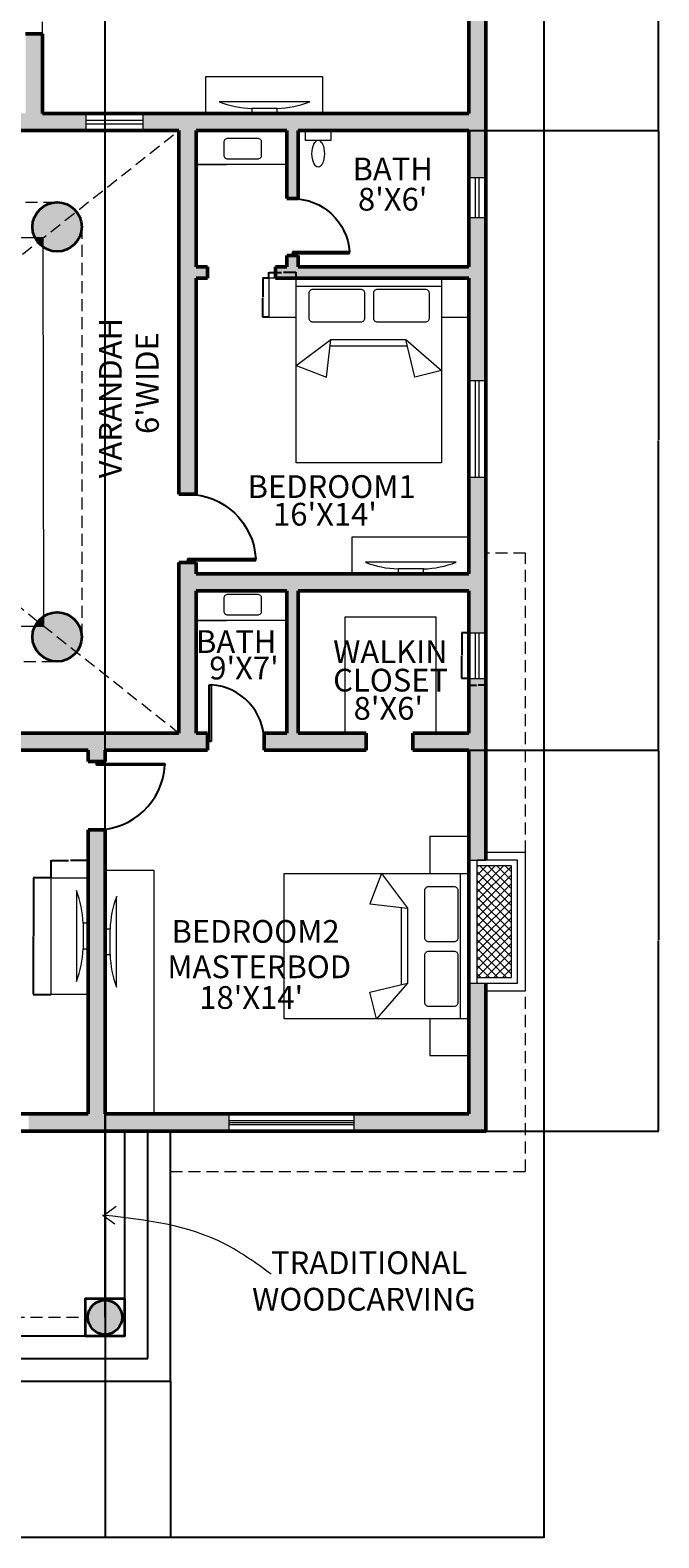
# Model space of a CAD drawing. Units: inches. Extents: x 2743 to 3669, y 1014 to 2282.
# Tile 3 of 5: x 3337 to 3669, y 1014 to 1810. Entities that reach past the tile are written whole.
import ezdxf

# ---------------------------------------------------------------- set-up
doc = ezdxf.new("R2010")
doc.units = ezdxf.units.IN
doc.linetypes.add('DASHED2', pattern=[9.525, 6.35, -3.175])
for name, color, linetype, lineweight in [('A-ANNO-DIMS', 2, 'Continuous', 18), ('A-ANNO-SYMB', 7, 'Continuous', 18), ('A-ANNO-TEXT', 4, 'Continuous', 18), ('A-AREA-IDEN', 4, 'Continuous', 18), ('A-COLS', 7, 'Continuous', 35), ('A-DOOR', 211, 'Continuous', 25), ('A-EQPM', 51, 'Continuous', 18), ('A-FLOR-CASE', 51, 'Continuous', 18), ('A-FLOR-STRS', 7, 'Continuous', 25), ('A-FURN', 111, 'Continuous', 18), ('A-GLAZ', 40, 'Continuous', 20), ('A-GLAZ-PATT', 8, 'Continuous', 13), ('A-ROOF', 7, 'Continuous', 20), ('A-ROOF-OVHD', 8, 'DASHED2', 18), ('A-WALL', 7, 'Continuous', 50), ('A-WALL-OVHD', 8, 'DASHED2', 18)]:
    doc.layers.add(name, color=color, linetype=linetype, lineweight=lineweight)
for name, color, linetype, lineweight, true_color in [('A-COLS-PATT', 47, 'Continuous', 13, 0x726c55), ('A-FLOR-FIXT', 11, 'Continuous', 18, 0xee778f), ('A-WALL-PATT', 47, 'Continuous', 13, 0x726c55)]:
    doc.layers.add(name, color=color, linetype=linetype, lineweight=lineweight, true_color=true_color)
doc.styles.get("Standard").update_dxf_attribs({"font": 'arial.ttf'})
doc.dimstyles.get("Standard").update_dxf_attribs({"dimtxt": 0.18, "dimasz": 0.18, "dimexe": 0.18, "dimexo": 0.0625, "dimgap": 0.09, "dimtad": 0, "dimtih": 1, "dimtoh": 1, "dimdec": 4, "dimzin": 0, "dimdsep": 46, "dimtxsty": 'Standard', "dimcen": 0.09, "dimadec": 0, "dimazin": 0, "dimtfac": 1, "dimtdec": 4, "dimtofl": 0, "dimtmove": 0, "dimatfit": 3, "dimfxl": 1, "dimtolj": 1, "dimtzin": 0, "dimarcsym": 0})

# ---------------------------------------------------------------- blocks, each defined once
blk = doc.blocks.new('DOOR-SINGLE-30IN')
for p, q in [((1, 0), (1, 30)), ((1, 30), (2, 30)), ((2, 30), (2, 0)), ((0, 0), (1, 0)), ((2, 0), (1, 0))]:
    blk.add_line(p, q)
blk.add_arc((0, 0.07), 30, 359.87254, 86.17759)
blk = doc.blocks.new('DOOR-SINGLE-36IN')
for p, q in [((1, 0), (1, 36)), ((1, 36), (2, 36)), ((2, 36), (2, 0)), ((0, 0), (1, 0)), ((2, 0), (1, 0))]:
    blk.add_line(p, q)
blk.add_arc((0, 0.06), 36, 359.91152, 86.81533)
blk = doc.blocks.new('WINDOW-24IN')
for p, q in [((0, 9), (0, 0)), ((24, 9), (24, 0)), ((0, 5.5), (24, 5.5)), ((0, 3.5), (24, 3.5))]:
    blk.add_line(p, q)
blk = doc.blocks.new('BED-DOUBLE')
for p, q in [((4.31, 76.75), (4.31, 0)), ((32.31, 57.96), (48.69, 76.75)), ((48.69, 76.75), (52.23, 62.72)), ((52.23, 62.72), (32.31, 57.96)), ((32.31, 18.34), (32.31, 57.96)), ((35.7, 17.95), (35.72, 58.78)), ((46.06, 0), (32.31, 18.34)), ((52.23, 16.05), (32.31, 18.34)), ((46.06, 0), (52.23, 16.05))]:
    blk.add_line(p, q)
blk.add_lwpolyline([(0, 76.75), (97.38, 76.75), (97.38, 0), (0, 0)], close=True)
for points in [[(7.76, 70.21), (21.16, 70.21, -0.414214), (23.16, 68.21), (23.16, 43, -0.414214), (21.16, 41), (7.76, 41, -0.414214), (5.76, 43), (5.76, 68.21, -0.414214)], [(7.76, 36.18), (21.16, 36.18, -0.414214), (23.16, 34.18), (23.16, 8.97, -0.414214), (21.16, 6.97), (7.76, 6.97, -0.414214), (5.76, 8.97), (5.76, 34.18, -0.414214)]]:
    blk.add_lwpolyline(points, format="xyb", close=True)
blk = doc.blocks.new('NIGHTSTAND')
blk.add_lwpolyline([(0, 0), (20.5, 0), (20.5, 19.45), (0, 19.45)], close=True)
blk = doc.blocks.new('NIGHTSTAND-NARROW')
for p, q in [((14.45, 20.49), (0, 20.49)), ((0, 20.49), (0, 0)), ((14.45, 0), (14.45, 20.49)), ((0, 0), (14.45, 0))]:
    blk.add_line(p, q)
blk = doc.blocks.new('WC')
blk.add_lwpolyline([(0, 13.38), (5.3, 13.38), (5.3, 0), (0, 0)], close=True)
blk.add_ellipse((12.29, 6.69), major_axis=(7.08, 0), ratio=0.464281)
blk = doc.blocks.new('BASIN')
for p, q in [((13.95, 48), (13.95, 0)), ((13.95, 0), (13.95, 16.09))]:
    blk.add_line(p, q)
blk.add_lwpolyline([(2, 34.47), (9.09, 34.47, -0.414214), (11.09, 32.47), (11.09, 16.89, -0.414214), (9.09, 14.89), (2, 14.89, -0.414214), (0, 16.89), (0, 32.47, -0.414214)], format="xyb", close=True)
blk = doc.blocks.new('TV-CONSOLE')
for p, q in [((0, 0), (0, 61.6)), ((0, 61.6), (19.53, 61.6)), ((19.53, 61.6), (19.53, 0)), ((13.42, 54.89), (13.42, 7)), ((19.53, 37.64), (16.89, 37.64)), ((16.89, 37.64), (16.89, 24.26)), ((16.89, 24.26), (19.53, 24.26)), ((19.53, 0), (0, 0))]:
    blk.add_line(p, q)
for centre, radius, start, end in [((-35.21, 36.13), 52.13, 1.66464, 21.09645), ((-35.14, 25.75), 52.05, 338.88993, 358.35791)]:
    blk.add_arc(centre, radius, start, end)
blk = doc.blocks.new('TV-SCREEN')
for p, q in [((6.11, 0), (6.11, 47.89)), ((2.64, 30.63), (0, 30.63)), ((2.64, 17.25), (2.64, 30.63)), ((0, 17.25), (2.64, 17.25))]:
    blk.add_line(p, q)
for centre, radius, start, end in [((54.67, 29.14), 52.05, 158.88993, 178.35791), ((54.74, 18.76), 52.13, 181.66464, 201.09645)]:
    blk.add_arc(centre, radius, start, end)
blk = doc.blocks.new('POST-COURTYARD')
blk.add_circle((13, 13), 13)
blk = doc.blocks.new('POST-SITOUT-OUTER')
blk.add_lwpolyline([(0, 0), (21.09, 0), (21.09, 19.48), (0, 19.48)], close=True)
blk.add_circle((10.55, 9.74), 9.06)
blk = doc.blocks.new('*D34')
at = {"layer": 'A-ANNO-DIMS', "color": 0, "lineweight": -2, "transparency": 16777216}
for p, q in [((3568.73, 1491.96), (3565.02, 1491.96)), ((3565.2, 1491.78), (3565.2, 1480.15)), ((3565.2, 1468.14), (3565.2, 1479.78)), ((3568.73, 1467.96), (3565.02, 1467.96))]:
    blk.add_line(p, q, dxfattribs=at)
at = {"layer": 'A-ANNO-DIMS', "color": 0, "transparency": 16777216}
for points in [[(3565.17, 1491.78), (3565.23, 1491.78), (3565.2, 1491.96)], [(3565.17, 1468.14), (3565.23, 1468.14), (3565.2, 1467.96)]]:
    blk.add_solid(points, dxfattribs=at)
at = {"layer": 'Defpoints', "color": 0, "transparency": 16777216}
for p in [(3565.2, 1491.96), (3568.8, 1491.96), (3568.8, 1467.96)]:
    blk.add_point(p, dxfattribs=at)
at = {"layer": 'A-ANNO-DIMS', "color": 0, "transparency": 16777216, "insert": (3565.2, 1479.96), "char_height": 0.18, "attachment_point": 5}
blk.add_mtext('\\A1;WINDOW 24 TYP.', dxfattribs=at)
blk = doc.blocks.new('*D35')
at = {"layer": 'A-ANNO-DIMS', "color": 0, "lineweight": -2, "transparency": 16777216}
for p, q in [((3568.8, 1467.9), (3568.8, 1464.18)), ((3568.98, 1464.36), (3572.84, 1464.36)), ((3577.62, 1464.36), (3573.75, 1464.36)), ((3577.8, 1467.9), (3577.8, 1464.18))]:
    blk.add_line(p, q, dxfattribs=at)
at = {"layer": 'A-ANNO-DIMS', "color": 0, "transparency": 16777216}
for points in [[(3568.98, 1464.39), (3568.98, 1464.33), (3568.8, 1464.36)], [(3577.62, 1464.39), (3577.62, 1464.33), (3577.8, 1464.36)]]:
    blk.add_solid(points, dxfattribs=at)
at = {"layer": 'Defpoints', "color": 0, "transparency": 16777216}
for p in [(3568.8, 1467.96), (3568.8, 1464.36), (3577.8, 1467.96)]:
    blk.add_point(p, dxfattribs=at)
at = {"layer": 'A-ANNO-DIMS', "color": 0, "transparency": 16777216, "insert": (3573.3, 1464.36), "char_height": 0.18, "attachment_point": 5}
blk.add_mtext('\\A1;9 TYP.', dxfattribs=at)
blk = doc.blocks.new('*D44')
at = {"layer": 'A-ANNO-DIMS', "color": 0, "lineweight": -2, "transparency": 16777216}
for p, q in [((3348.2, 1362.64), (3338.85, 1362.64)), ((3339.03, 1362.46), (3339.03, 1332.03)), ((3339.03, 1301.22), (3339.03, 1331.66)), ((3348.2, 1301.04), (3338.85, 1301.04))]:
    blk.add_line(p, q, dxfattribs=at)
at = {"layer": 'A-ANNO-DIMS', "color": 0, "transparency": 16777216}
for points in [[(3339, 1362.46), (3339.06, 1362.46), (3339.03, 1362.64)], [(3339, 1301.22), (3339.06, 1301.22), (3339.03, 1301.04)]]:
    blk.add_solid(points, dxfattribs=at)
at = {"layer": 'Defpoints', "color": 0, "transparency": 16777216}
for p in [(3339.03, 1362.64), (3348.27, 1362.64), (3348.27, 1301.04)]:
    blk.add_point(p, dxfattribs=at)
at = {"layer": 'A-ANNO-DIMS', "color": 0, "transparency": 16777216, "insert": (3339.03, 1331.84), "char_height": 0.18, "attachment_point": 5}
blk.add_mtext('\\A1;CONSOLE 62 TYP.', dxfattribs=at)
blk = doc.blocks.new('*D45')
at = {"layer": 'A-ANNO-DIMS', "color": 0, "lineweight": -2, "transparency": 16777216}
for p, q in [((3348.27, 1362.71), (3348.27, 1372.06)), ((3348.45, 1371.88), (3357.5, 1371.88)), ((3367.62, 1371.88), (3358.56, 1371.88)), ((3367.8, 1362.71), (3367.8, 1372.06))]:
    blk.add_line(p, q, dxfattribs=at)
at = {"layer": 'A-ANNO-DIMS', "color": 0, "transparency": 16777216}
for points in [[(3348.45, 1371.91), (3348.45, 1371.85), (3348.27, 1371.88)], [(3367.62, 1371.91), (3367.62, 1371.85), (3367.8, 1371.88)]]:
    blk.add_solid(points, dxfattribs=at)
at = {"layer": 'Defpoints', "color": 0, "transparency": 16777216}
for p in [(3367.8, 1371.88), (3348.27, 1362.64), (3367.8, 1362.64)]:
    blk.add_point(p, dxfattribs=at)
at = {"layer": 'A-ANNO-DIMS', "color": 0, "transparency": 16777216, "insert": (3358.03, 1371.88), "char_height": 0.18, "attachment_point": 5}
blk.add_mtext('\\A1;20 TYP.', dxfattribs=at)
blk = doc.blocks.new('*D52')
at = {"layer": 'A-ANNO-DIMS', "color": 0, "lineweight": -2, "transparency": 16777216}
for p, q in [((3463.09, 1679.09), (3459.9, 1679.09)), ((3460.08, 1678.91), (3460.08, 1669.03)), ((3460.08, 1658.78), (3460.08, 1668.66)), ((3463.09, 1658.6), (3459.9, 1658.6))]:
    blk.add_line(p, q, dxfattribs=at)
at = {"layer": 'A-ANNO-DIMS', "color": 0, "transparency": 16777216}
for points in [[(3460.05, 1678.91), (3460.11, 1678.91), (3460.08, 1679.09)], [(3460.05, 1658.78), (3460.11, 1658.78), (3460.08, 1658.6)]]:
    blk.add_solid(points, dxfattribs=at)
at = {"layer": 'Defpoints', "color": 0, "transparency": 16777216}
for p in [(3460.08, 1679.09), (3463.15, 1679.09), (3463.15, 1658.6)]:
    blk.add_point(p, dxfattribs=at)
at = {"layer": 'A-ANNO-DIMS', "color": 0, "transparency": 16777216, "insert": (3460.08, 1668.85), "char_height": 0.18, "attachment_point": 5}
blk.add_mtext('\\A1;STAND 20 TYP.', dxfattribs=at)
blk = doc.blocks.new('*D53')
at = {"layer": 'A-ANNO-DIMS', "color": 0, "lineweight": -2, "transparency": 16777216}
for p, q in [((3463.15, 1679.16), (3463.15, 1682.35)), ((3463.33, 1682.17), (3469.86, 1682.17)), ((3477.42, 1682.17), (3470.9, 1682.17)), ((3477.6, 1679.16), (3477.6, 1682.35))]:
    blk.add_line(p, q, dxfattribs=at)
at = {"layer": 'A-ANNO-DIMS', "color": 0, "transparency": 16777216}
for points in [[(3463.33, 1682.2), (3463.33, 1682.14), (3463.15, 1682.17)], [(3477.42, 1682.2), (3477.42, 1682.14), (3477.6, 1682.17)]]:
    blk.add_solid(points, dxfattribs=at)
at = {"layer": 'Defpoints', "color": 0, "transparency": 16777216}
for p in [(3463.15, 1679.09), (3477.6, 1682.17), (3477.6, 1679.09)]:
    blk.add_point(p, dxfattribs=at)
at = {"layer": 'A-ANNO-DIMS', "color": 0, "transparency": 16777216, "insert": (3470.38, 1682.17), "char_height": 0.18, "attachment_point": 5}
blk.add_mtext('\\A1;14 TYP.', dxfattribs=at)
blk = doc.blocks.new('*D62')
at = {"layer": 'A-ANNO-DIMS', "color": 0, "lineweight": -2, "transparency": 16777216}
for p, q in [((3608.38, 1899.55), (3608.38, 1014.41)), ((2803.91, 1765.52), (2803.91, 1014.41)), ((2804.09, 1014.59), (3205.75, 1014.59)), ((3608.2, 1014.59), (3206.54, 1014.59))]:
    blk.add_line(p, q, dxfattribs=at)
at = {"layer": 'A-ANNO-DIMS', "color": 0, "transparency": 16777216}
for points in [[(2804.09, 1014.62), (2804.09, 1014.56), (2803.91, 1014.59)], [(3608.2, 1014.62), (3608.2, 1014.56), (3608.38, 1014.59)]]:
    blk.add_solid(points, dxfattribs=at)
at = {"layer": 'Defpoints', "color": 0, "transparency": 16777216}
for p in [(3608.38, 1899.61), (2803.91, 1765.58), (3608.38, 1014.59)]:
    blk.add_point(p, dxfattribs=at)
at = {"layer": 'A-ANNO-DIMS', "color": 0, "transparency": 16777216, "insert": (3206.15, 1014.59), "char_height": 0.18, "attachment_point": 5}
blk.add_mtext('\\A1;804.5', dxfattribs=at)
blk = doc.blocks.new('*D67')
at = {"layer": 'A-ANNO-DIMS', "color": 0, "lineweight": -2, "transparency": 16777216}
for p, q in [((3568.86, 1430.09), (3669.11, 1430.09)), ((3668.93, 1429.91), (3668.93, 1329.78)), ((3668.93, 1229.27), (3668.93, 1329.41)), ((3577.86, 1229.09), (3669.11, 1229.09))]:
    blk.add_line(p, q, dxfattribs=at)
at = {"layer": 'A-ANNO-DIMS', "color": 0, "transparency": 16777216}
for points in [[(3668.9, 1429.91), (3668.96, 1429.91), (3668.93, 1430.09)], [(3668.9, 1229.27), (3668.96, 1229.27), (3668.93, 1229.09)]]:
    blk.add_solid(points, dxfattribs=at)
at = {"layer": 'Defpoints', "color": 0, "transparency": 16777216}
for p in [(3568.8, 1430.09), (3668.93, 1430.09), (3577.8, 1229.09)]:
    blk.add_point(p, dxfattribs=at)
at = {"layer": 'A-ANNO-DIMS', "color": 0, "transparency": 16777216, "insert": (3668.93, 1329.59), "char_height": 0.18, "attachment_point": 5}
blk.add_mtext('\\A1;201', dxfattribs=at)
blk = doc.blocks.new('*D68')
at = {"layer": 'A-ANNO-DIMS', "color": 0, "lineweight": -2, "transparency": 16777216}
for p, q in [((3568.86, 1757.09), (3669.11, 1757.09)), ((3668.93, 1756.91), (3668.93, 1593.78)), ((3668.93, 1430.27), (3668.93, 1593.41)), ((3568.86, 1430.09), (3669.11, 1430.09))]:
    blk.add_line(p, q, dxfattribs=at)
at = {"layer": 'A-ANNO-DIMS', "color": 0, "transparency": 16777216}
for points in [[(3668.9, 1756.91), (3668.96, 1756.91), (3668.93, 1757.09)], [(3668.9, 1430.27), (3668.96, 1430.27), (3668.93, 1430.09)]]:
    blk.add_solid(points, dxfattribs=at)
at = {"layer": 'Defpoints', "color": 0, "transparency": 16777216}
for p in [(3568.8, 1757.09), (3668.93, 1757.09), (3568.8, 1430.09)]:
    blk.add_point(p, dxfattribs=at)
at = {"layer": 'A-ANNO-DIMS', "color": 0, "transparency": 16777216, "insert": (3668.93, 1593.59), "char_height": 0.18, "attachment_point": 5}
blk.add_mtext('\\A1;327', dxfattribs=at)
blk = doc.blocks.new('*D69')
at = {"layer": 'A-ANNO-DIMS', "color": 0, "lineweight": -2, "transparency": 16777216}
for p, q in [((3568.86, 1958.09), (3669.11, 1958.09)), ((3668.93, 1957.91), (3668.93, 1857.78)), ((3668.93, 1757.27), (3668.93, 1857.41)), ((3568.86, 1757.09), (3669.11, 1757.09))]:
    blk.add_line(p, q, dxfattribs=at)
at = {"layer": 'A-ANNO-DIMS', "color": 0, "transparency": 16777216}
for points in [[(3668.9, 1957.91), (3668.96, 1957.91), (3668.93, 1958.09)], [(3668.9, 1757.27), (3668.96, 1757.27), (3668.93, 1757.09)]]:
    blk.add_solid(points, dxfattribs=at)
at = {"layer": 'Defpoints', "color": 0, "transparency": 16777216}
for p in [(3568.8, 1958.09), (3668.93, 1958.09), (3568.8, 1757.09)]:
    blk.add_point(p, dxfattribs=at)
at = {"layer": 'A-ANNO-DIMS', "color": 0, "transparency": 16777216, "insert": (3668.93, 1857.59), "char_height": 0.18, "attachment_point": 5}
blk.add_mtext('\\A1;201', dxfattribs=at)
blk = doc.blocks.new('*D74')
at = {"layer": 'A-ANNO-DIMS', "color": 0, "lineweight": -2, "transparency": 16777216}
for p, q in [((3052.8, 1238.03), (3052.8, 1014.41)), ((3376.8, 1238.03), (3376.8, 1014.41)), ((3052.98, 1014.59), (3214.51, 1014.59)), ((3376.62, 1014.59), (3215.08, 1014.59))]:
    blk.add_line(p, q, dxfattribs=at)
at = {"layer": 'A-ANNO-DIMS', "color": 0, "transparency": 16777216}
for points in [[(3052.98, 1014.62), (3052.98, 1014.56), (3052.8, 1014.59)], [(3376.62, 1014.62), (3376.62, 1014.56), (3376.8, 1014.59)]]:
    blk.add_solid(points, dxfattribs=at)
at = {"layer": 'Defpoints', "color": 0, "transparency": 16777216}
for p in [(3052.8, 1238.09), (3376.8, 1238.09), (3376.8, 1014.59)]:
    blk.add_point(p, dxfattribs=at)
at = {"layer": 'A-ANNO-DIMS', "color": 0, "transparency": 16777216, "insert": (3214.8, 1014.59), "char_height": 0.18, "attachment_point": 5}
blk.add_mtext('\\A1;324', dxfattribs=at)
blk = doc.blocks.new('*D75')
at = {"layer": 'A-ANNO-DIMS', "color": 0, "lineweight": -2, "transparency": 16777216}
for p, q in [((3018.3, 1097.03), (3018.3, 1014.41)), ((3411.3, 1097.03), (3411.3, 1014.41)), ((3018.48, 1014.59), (3214.51, 1014.59)), ((3411.12, 1014.59), (3215.09, 1014.59))]:
    blk.add_line(p, q, dxfattribs=at)
at = {"layer": 'A-ANNO-DIMS', "color": 0, "transparency": 16777216}
for points in [[(3018.48, 1014.62), (3018.48, 1014.56), (3018.3, 1014.59)], [(3411.12, 1014.62), (3411.12, 1014.56), (3411.3, 1014.59)]]:
    blk.add_solid(points, dxfattribs=at)
at = {"layer": 'Defpoints', "color": 0, "transparency": 16777216}
for p in [(3018.3, 1097.09), (3411.3, 1097.09), (3411.3, 1014.59)]:
    blk.add_point(p, dxfattribs=at)
at = {"layer": 'A-ANNO-DIMS', "color": 0, "transparency": 16777216, "insert": (3214.8, 1014.59), "char_height": 0.18, "attachment_point": 5}
blk.add_mtext('\\A1;393', dxfattribs=at)
blk = doc.blocks.new('*D78')
at = {"layer": 'A-ANNO-DIMS', "color": 0, "lineweight": -2, "transparency": 16777216}
for p, q in [((3271.8, 1130.9), (3271.8, 2281.6)), ((3271.98, 2281.42), (3323.82, 2281.42)), ((3376.57, 2281.42), (3324.73, 2281.42)), ((3376.75, 1130.9), (3376.75, 2281.6))]:
    blk.add_line(p, q, dxfattribs=at)
at = {"layer": 'A-ANNO-DIMS', "color": 0, "transparency": 16777216}
for points in [[(3271.98, 2281.45), (3271.98, 2281.39), (3271.8, 2281.42)], [(3376.57, 2281.45), (3376.57, 2281.39), (3376.75, 2281.42)]]:
    blk.add_solid(points, dxfattribs=at)
at = {"layer": 'Defpoints', "color": 0, "transparency": 16777216}
for p in [(3376.75, 2281.42), (3271.8, 1130.83), (3376.75, 1130.83)]:
    blk.add_point(p, dxfattribs=at)
at = {"layer": 'A-ANNO-DIMS', "color": 0, "transparency": 16777216, "insert": (3324.27, 2281.42), "char_height": 0.18, "attachment_point": 5}
blk.add_mtext('\\A1;104.95', dxfattribs=at)

msp = doc.modelspace()

# ---------------------------------------------------------------- hatches: boundary and pattern name
at = {"layer": 'A-COLS-PATT'}
h = msp.add_hatch(color=256, dxfattribs=at)
h.dxf.hatch_style = 1
h.paths.add_polyline_path([(3338.466, 1706.206, 0.115947), (3339.827, 1700.414), (3344.132, 1700.404), (3361.661, 1714.271, 0.7110205)])
h = msp.add_hatch(color=256, dxfattribs=at)
h.dxf.hatch_style = 1
h.paths.add_polyline_path([(3364.466, 1706.206, 0.1688931), (3361.661, 1714.271), (3344.132, 1700.404), (3344.141, 1695.466, 0.6026199)])
h = msp.add_hatch(color=256, dxfattribs=at)
h.dxf.hatch_style = 1
h.paths.add_polyline_path([(3344.132, 1700.404), (3339.827, 1700.414, 0.0519292), (3341.27, 1698.14)])
h = msp.add_hatch(color=256, dxfattribs=at)
h.dxf.hatch_style = 1
h.paths.add_polyline_path([(3344.132, 1700.404), (3341.27, 1698.14, 0.0758855), (3344.141, 1695.466)])
h = msp.add_hatch(color=256, dxfattribs=at)
h.dxf.hatch_style = 1
h.paths.add_polyline_path([(3341.341, 1497.992, 0.0572464), (3339.756, 1495.484), (3344.492, 1495.499)])
h = msp.add_hatch(color=256, dxfattribs=at)
h.dxf.hatch_style = 1
h.paths.add_polyline_path([(3344.483, 1500.803, 0.0816056), (3341.341, 1497.992), (3344.492, 1495.499)])
h = msp.add_hatch(color=256, dxfattribs=at)
h.dxf.hatch_style = 1
h.paths.add_polyline_path([(3361.732, 1481.862, 0.1666401), (3364.466, 1489.837, 0.591934), (3344.483, 1500.803), (3344.492, 1495.499)])
h = msp.add_hatch(color=256, dxfattribs=at)
h.dxf.hatch_style = 1
h.paths.add_polyline_path([(3344.492, 1495.499), (3339.756, 1495.484, 0.1127962), (3338.466, 1489.837, 0.7143248), (3361.732, 1481.862)])
h = msp.add_hatch(color=256, dxfattribs=at)
h.dxf.hatch_style = 1
h.paths.add_polyline_path([(3367.688, 1130.835, 1), (3385.814, 1130.835, 1)])
at = {"layer": 'A-GLAZ-PATT'}
h = msp.add_hatch(dxfattribs=at)
h.set_pattern_fill('ANSI37', color=256)
h.paths.add_polyline_path([(3591.296, 1369.044), (3573.296, 1369.044), (3573.296, 1310.044), (3591.296, 1310.044)])
at = {"layer": 'A-WALL-PATT'}
h = msp.add_hatch(color=256, dxfattribs=at)
h.dxf.hatch_style = 1
h.paths.add_polyline_path([(3415.796, 1757.094), (3415.796, 1565.094), (3424.796, 1565.094), (3424.796, 1679.094), (3430.796, 1679.094), (3430.796, 1685.094), (3424.796, 1685.094), (3424.796, 1757.094), (3472.796, 1757.094), (3472.796, 1721.094), (3478.796, 1721.094), (3478.796, 1757.094), (3568.796, 1757.094), (3568.796, 1732.183), (3577.796, 1732.183), (3577.796, 1824.222), (3568.796, 1824.222), (3568.796, 1766.094), (3396.681, 1766.094), (3396.681, 1757.094)])
h = msp.add_hatch(color=256, dxfattribs=at)
h.dxf.hatch_style = 1
h.paths.add_polyline_path([(3312.269, 1766.094), (3312.269, 1757.094), (3366.681, 1757.094), (3366.681, 1766.094), (3343.796, 1766.094), (3343.796, 1808.094), (3334.796, 1808.094), (3334.796, 1766.094)])
h = msp.add_hatch(color=256, dxfattribs=at)
h.dxf.hatch_style = 1
h.paths.add_polyline_path([(3577.796, 1711.183), (3568.796, 1711.183), (3568.796, 1685.094), (3478.796, 1685.094), (3478.796, 1691.094), (3472.796, 1691.094), (3472.796, 1685.094), (3466.796, 1685.094), (3466.796, 1679.094), (3477.6, 1679.094), (3554.349, 1679.094), (3568.796, 1679.094), (3568.796, 1658.6), (3568.796, 1625.145), (3577.796, 1625.145)], flags=17)
h = msp.add_hatch(color=256, dxfattribs=at)
h.dxf.hatch_style = 1
h.paths.add_polyline_path([(3568.796, 1514.094), (3568.796, 1491.964), (3577.796, 1491.964), (3577.796, 1574.145), (3568.796, 1574.145), (3568.796, 1523.094), (3507.198, 1523.094), (3424.796, 1523.094), (3424.796, 1529.094), (3415.796, 1529.094), (3415.796, 1439.094), (3326.438, 1439.094), (3326.438, 1430.094), (3367.796, 1430.094), (3367.796, 1424.094), (3376.796, 1424.094), (3376.796, 1430.094), (3430.796, 1430.094), (3430.796, 1439.094), (3424.796, 1439.094), (3424.796, 1514.094), (3472.796, 1514.094), (3472.796, 1439.094), (3460.796, 1439.094), (3460.796, 1430.094), (3514.579, 1430.094), (3514.579, 1439.094), (3478.796, 1439.094), (3478.796, 1514.094)])
h = msp.add_hatch(color=256, dxfattribs=at)
h.dxf.hatch_style = 1
h.paths.add_polyline_path([(3568.796, 1430.094), (3568.796, 1372.069), (3577.796, 1372.069), (3577.796, 1467.964), (3568.796, 1467.964), (3568.796, 1439.094), (3539.188, 1439.094), (3539.188, 1430.094)])
h = msp.add_hatch(color=256, dxfattribs=at)
h.dxf.hatch_style = 1
h.paths.add_polyline_path([(3336.421, 1238.094), (3336.421, 1229.094), (3442.044, 1229.094), (3442.044, 1238.094), (3376.796, 1238.094), (3376.796, 1366.758), (3376.796, 1388.094), (3367.796, 1388.094), (3367.796, 1238.094)])
h = msp.add_hatch(color=256, dxfattribs=at)
h.dxf.hatch_style = 1
h.paths.add_polyline_path([(3577.796, 1229.094), (3577.796, 1307.044), (3568.796, 1307.044), (3568.796, 1288.306), (3568.796, 1268.859), (3568.796, 1238.094), (3508.044, 1238.094), (3508.044, 1229.094)])

# ---------------------------------------------------------------- linework, layer by layer
at = {"layer": 'A-ANNO-SYMB'}
for p, q in [((3376.022, 1184.568), (3382.632, 1189.367)), ((3375.657, 1184.604), (3381.997, 1180.074))]:
    msp.add_line(p, q, dxfattribs=at)
msp.add_open_spline([(3464.392, 1153.561), (3456.457, 1159.355), (3430.922, 1178.001), (3397.907, 1182.411), (3376.022, 1184.568), (3375.657, 1184.604)], degree=3, knots=[0, 0, 0, 0, 29.2551679, 94.1473437, 95.246917, 95.246917, 95.246917, 95.246917], dxfattribs=at)
at = {"layer": 'A-FLOR-CASE'}
for p, q in [((3503.538, 1439.094), (3503.538, 1500.431)), ((3503.538, 1500.431), (3551.337, 1500.431)), ((3551.337, 1500.431), (3551.337, 1439.094))]:
    msp.add_line(p, q, dxfattribs=at)
msp.add_lwpolyline([(3402.509, 1238.094), (3376.796, 1238.094), (3376.796, 1366.758), (3402.509, 1366.758)], close=True, dxfattribs=at)
at = {"layer": 'A-FLOR-STRS'}
for p, q in [((3387.296, 1121.094), (3387.296, 1229.094)), ((3399.296, 1109.094), (3399.296, 1229.094)), ((3411.296, 1097.094), (3411.296, 1229.094)), ((3042.296, 1121.094), (3387.296, 1121.094)), ((3280.796, 1109.094), (3399.296, 1109.094)), ((3280.796, 1097.094), (3411.296, 1097.094))]:
    msp.add_line(p, q, dxfattribs=at)
at = {"layer": 'A-GLAZ'}
for p, q in [((3366.681, 1766.094), (3366.681, 1757.094)), ((3366.681, 1762.594), (3396.681, 1762.594)), ((3366.681, 1760.594), (3396.681, 1760.594)), ((3396.681, 1766.094), (3396.681, 1757.094)), ((3568.796, 1732.183), (3577.796, 1732.183)), ((3572.296, 1711.183), (3572.296, 1732.183)), ((3574.296, 1711.183), (3574.296, 1732.183)), ((3568.796, 1711.183), (3577.796, 1711.183)), ((3568.796, 1625.145), (3577.796, 1625.145)), ((3572.296, 1574.145), (3572.296, 1625.145)), ((3574.296, 1574.145), (3574.296, 1625.145)), ((3568.796, 1574.145), (3577.796, 1574.145)), ((3568.796, 1372.069), (3577.796, 1372.069)), ((3573.296, 1307.044), (3573.296, 1372.069)), ((3594.531, 1372.069), (3573.296, 1372.069)), ((3591.296, 1369.044), (3573.296, 1369.044)), ((3591.296, 1310.044), (3591.296, 1369.044)), ((3594.531, 1307.044), (3594.531, 1372.069)), ((3568.796, 1307.044), (3577.796, 1307.044)), ((3573.296, 1310.044), (3591.296, 1310.044)), ((3577.796, 1307.044), (3594.531, 1307.044)), ((3442.044, 1238.094), (3442.044, 1229.094)), ((3442.044, 1234.594), (3508.044, 1234.594)), ((3442.044, 1233.594), (3508.044, 1233.594)), ((3508.044, 1238.094), (3508.044, 1229.094)), ((3442.044, 1232.594), (3508.044, 1232.594))]:
    msp.add_line(p, q, dxfattribs=at)
at = {"layer": 'A-ROOF'}
for p, q in [((3344.132, 1700.404), (3084.483, 1701.002)), ((3344.492, 1495.499), (3344.132, 1700.404)), ((3084.008, 1494.635), (3344.492, 1495.499)), ((3598.796, 1376.044), (3577.796, 1376.044)), ((3598.796, 1303.044), (3598.796, 1376.044)), ((3577.796, 1303.044), (3598.796, 1303.044))]:
    msp.add_line(p, q, dxfattribs=at)
at = {"layer": 'A-ROOF-OVHD'}
for p, q in [((3258.517, 1632.679), (3415.796, 1757.094)), ((3077.548, 1719.664), (3351.487, 1719.206)), ((3364.466, 1706.206), (3364.466, 1489.837)), ((3261.659, 1561.024), (3415.796, 1439.094)), ((3598.796, 1534.038), (3577.796, 1534.038)), ((3598.796, 1376.044), (3598.796, 1534.038)), ((3076.759, 1475.9), (3351.466, 1476.837)), ((3598.796, 1207.768), (3598.796, 1303.044)), ((3376.751, 1139.898), (3376.751, 1229.094)), ((3411.296, 1207.768), (3598.796, 1207.768)), ((3280.201, 1130.835), (3367.688, 1130.835))]:
    msp.add_line(p, q, dxfattribs=at)
at = {"layer": 'A-WALL'}
for p, q in [((3568.796, 1838.222), (3568.796, 1766.094)), ((3334.796, 1808.094), (3343.796, 1808.094)), ((3343.796, 1766.094), (3343.796, 1808.094)), ((3343.796, 1766.094), (3568.796, 1766.094)), ((3244.796, 1757.094), (3415.796, 1757.094)), ((3415.796, 1757.094), (3415.796, 1565.094)), ((3424.796, 1757.094), (3424.796, 1685.094)), ((3424.796, 1757.094), (3472.796, 1757.094)), ((3472.796, 1757.094), (3472.796, 1721.094)), ((3478.796, 1757.094), (3478.796, 1721.094)), ((3478.796, 1757.094), (3568.796, 1757.094)), ((3568.796, 1757.094), (3568.796, 1685.094)), ((3472.796, 1721.094), (3478.796, 1721.094)), ((3472.796, 1685.094), (3472.796, 1691.094)), ((3472.796, 1691.094), (3478.796, 1691.094)), ((3472.796, 1691.094), (3472.796, 1685.094)), ((3478.796, 1691.094), (3478.796, 1685.094)), ((3424.796, 1685.094), (3430.796, 1685.094)), ((3424.796, 1679.094), (3430.796, 1679.094)), ((3424.796, 1679.094), (3424.796, 1565.094)), ((3430.796, 1685.094), (3430.796, 1679.094)), ((3466.796, 1685.094), (3466.796, 1679.094)), ((3466.796, 1685.094), (3472.796, 1685.094)), ((3466.796, 1679.094), (3568.796, 1679.094)), ((3478.796, 1685.094), (3568.796, 1685.094)), ((3568.796, 1679.094), (3568.796, 1523.094)), ((3424.796, 1565.094), (3415.796, 1565.094)), ((3424.796, 1529.094), (3415.796, 1529.094)), ((3415.796, 1529.094), (3415.796, 1439.094)), ((3424.796, 1529.094), (3424.796, 1523.094)), ((3424.796, 1523.094), (3568.796, 1523.094)), ((3424.796, 1514.094), (3472.796, 1514.094)), ((3424.796, 1514.094), (3424.796, 1439.094)), ((3472.796, 1514.094), (3472.796, 1439.094)), ((3478.796, 1514.094), (3478.796, 1439.094)), ((3478.796, 1514.094), (3568.796, 1514.094)), ((3568.796, 1514.094), (3568.796, 1439.094)), ((3415.796, 1439.094), (3244.796, 1439.094)), ((3430.796, 1439.094), (3424.796, 1439.094)), ((3430.796, 1439.094), (3430.796, 1430.094)), ((3472.796, 1439.094), (3460.796, 1439.094)), ((3460.796, 1439.094), (3460.796, 1430.094)), ((3514.579, 1439.094), (3478.796, 1439.094)), ((3514.579, 1439.094), (3514.579, 1430.094)), ((3568.796, 1439.094), (3539.188, 1439.094)), ((3539.188, 1439.094), (3539.188, 1430.094)), ((3367.796, 1430.094), (3244.796, 1430.094)), ((3367.796, 1430.094), (3367.796, 1424.094)), ((3376.796, 1430.094), (3376.796, 1424.094)), ((3430.796, 1430.094), (3376.796, 1430.094)), ((3514.579, 1430.094), (3460.796, 1430.094)), ((3568.796, 1430.094), (3539.188, 1430.094)), ((3568.796, 1430.094), (3568.796, 1238.094)), ((3367.796, 1424.094), (3376.796, 1424.094)), ((3367.796, 1388.094), (3376.796, 1388.094)), ((3367.796, 1388.094), (3367.796, 1238.094)), ((3376.796, 1388.094), (3376.796, 1238.094)), ((3367.796, 1238.094), (3244.796, 1238.094)), ((3568.796, 1238.094), (3376.796, 1238.094))]:
    msp.add_line(p, q, dxfattribs=at)
for points in [[(3577.796, 1824.222), (3577.796, 1372.069)], [(3577.796, 1307.044), (3577.796, 1229.094), (3244.796, 1229.094)]]:
    msp.add_lwpolyline(points, dxfattribs=at)
at = {"layer": 'A-WALL-OVHD'}
msp.add_line((3343.796, 1808.094), (3343.796, 1916.094), dxfattribs=at)

# ---------------------------------------------------------------- block references
at = {"layer": 'A-COLS'}
for name, p in [('POST-COURTYARD', (3338.466, 1693.206)), ('POST-COURTYARD', (3338.466, 1476.838)), ('POST-SITOUT-OUTER', (3366.206, 1121.094))]:
    msp.add_blockref(name, p, dxfattribs=at)
at = {"layer": 'A-DOOR', "extrusion": (0, 0, -1), "zscale": -1}
for name, p, rotation in [('DOOR-SINGLE-30IN', (-3475.796, 1691.094), 89.9999999999992), ('DOOR-SINGLE-36IN', (-3420.296, 1529.094), 90.00000000000246)]:
    msp.add_blockref(name, p, dxfattribs=dict(at, rotation=rotation))
at = {"layer": 'A-DOOR'}
msp.add_blockref('DOOR-SINGLE-30IN', (3430.796, 1434.594), dxfattribs=at)
at = {"layer": 'A-DOOR', "rotation": 270.0000000000004}
msp.add_blockref('DOOR-SINGLE-36IN', (3372.296, 1424.095), dxfattribs=at)
at = {"layer": 'A-EQPM'}
for p, rotation in [((3429.947, 1785.625), 269.9999999999989), ((3507.198, 1542.625), 269.999999999999)]:
    msp.add_blockref('TV-CONSOLE', p, dxfattribs=dict(at, rotation=rotation))
for name, p in [('TV-CONSOLE', (3348.266, 1301.045)), ('TV-SCREEN', (3376.796, 1304.969))]:
    msp.add_blockref(name, p, dxfattribs=at)
at = {"layer": 'A-FLOR-FIXT'}
for name, p, rotation in [('BASIN', (3424.796, 1753.045), 270.0000000000017), ('WC', (3482.609, 1757.095), 269.9999999999915), ('BASIN', (3424.796, 1512.355), 270.0000000000007)]:
    msp.add_blockref(name, p, dxfattribs=dict(at, rotation=rotation))
at = {"layer": 'A-FURN'}
for p in [(3463.152, 1658.6), (3554.349, 1658.6)]:
    msp.add_blockref('NIGHTSTAND-NARROW', p, dxfattribs=at)
for name, p, rotation in [('BED-DOUBLE', (3477.6, 1679.095), 270.0000000000015), ('NIGHTSTAND', (3568.797, 1384.503), 180), ('BED-DOUBLE', (3568.797, 1365.055), 180), ('NIGHTSTAND', (3568.797, 1288.306), 180)]:
    msp.add_blockref(name, p, dxfattribs=dict(at, rotation=rotation))
at = {"layer": 'A-GLAZ', "rotation": 89.9999999999992}
msp.add_blockref('WINDOW-24IN', (3577.797, 1467.964), dxfattribs=at)

# ---------------------------------------------------------------- texts
at = {"layer": 'A-ANNO-TEXT'}
for tag, p in [('TRADITIONAL', (3464.392, 1153.561)), ('WOODCARVING', (3454.387, 1134.337))]:
    msp.add_attdef(tag, p, '', height=12, dxfattribs=at)
at = {"layer": 'A-AREA-IDEN'}
for tag, p in [('BATH', (3507.421, 1730.766)), ("8'X6'", (3510.287, 1714.779)), ('BEDROOM1', (3452.022, 1563.16)), ("16'X14'", (3465.476, 1548.565)), ('BATH', (3424.796, 1481.378)), ('WALKIN', (3497.198, 1476.06)), ("9'X7'", (3431.796, 1467.397)), ('CLOSET', (3497.198, 1461.015)), ("8'X6'", (3507.997, 1446.122)), ('BEDROOM2', (3411.867, 1328.425)), ('MASTERBOD', (3409.673, 1309.748)), ("18'X14'", (3426.514, 1293.557))]:
    msp.add_attdef(tag, p, '', height=12, dxfattribs=at)
for tag, p, rotation in [('VARANDAH', (3385.508, 1573.482), 89.904183), ("6'WIDE", (3405.178, 1596.927), 90.261085)]:
    msp.add_attdef(tag, p, '', height=12, rotation=rotation, dxfattribs=at)

# ---------------------------------------------------------------- dimensions: what is measured, and where the dimension line sits
at = {"layer": 'A-ANNO-DIMS'}
for base, p1, p2, override, picture, middle in [((3376.7513, 2281.4212), (3271.7965, 1130.8347), (3376.7513, 1130.8347), {"dimdec": 2, "dimlfac": 1, "dimrnd": 0, "dimzin": 0, "dimdsep": 46, "dimlunit": 2}, '*D78', (3324.2739, 2281.4212)), ((3608.383, 1014.589), (2803.91, 1765.581), (3608.383, 1899.608), {"dimdec": 1, "dimlfac": 1, "dimrnd": 0, "dimzin": 0, "dimdsep": 46, "dimlunit": 2}, '*D62', (3206.146, 1014.589)), ((3376.796, 1014.589), (3052.796, 1238.094), (3376.796, 1238.094), {"dimdec": 0, "dimlfac": 1, "dimrnd": 0, "dimzin": 0, "dimdsep": 46, "dimlunit": 2}, '*D74', (3214.796, 1014.589)), ((3411.296, 1014.589), (3018.296, 1097.094), (3411.296, 1097.094), {"dimdec": 0, "dimlfac": 1, "dimrnd": 0, "dimzin": 0, "dimdsep": 46, "dimlunit": 2}, '*D75', (3214.796, 1014.589))]:
    dim = msp.add_linear_dim(base=base, p1=p1, p2=p2, dimstyle='Standard', override=override, dxfattribs=at)
    dim.commit()
    dim.dimension.update_dxf_attribs({"geometry": picture, "text_midpoint": middle})
for base, p1, p2, picture, middle in [((3668.933, 1958.094), (3568.796, 1757.094), (3568.796, 1958.094), '*D69', (3668.933, 1857.594)), ((3668.933, 1757.094), (3568.796, 1430.094), (3568.796, 1757.094), '*D68', (3668.933, 1593.594)), ((3668.933, 1430.094), (3577.796, 1229.094), (3568.796, 1430.094), '*D67', (3668.933, 1329.594))]:
    dim = msp.add_linear_dim(base=base, p1=p1, p2=p2, angle=90, dimstyle='Standard', override={"dimdec": 0, "dimlfac": 1, "dimrnd": 0, "dimzin": 0, "dimdsep": 46, "dimlunit": 2}, dxfattribs=at)
    dim.commit()
    dim.dimension.update_dxf_attribs({"geometry": picture, "text_midpoint": middle})
for base, p1, p2, angle, text, picture, middle in [((3460.078, 1679.094), (3463.152, 1658.6), (3463.152, 1679.094), 90, 'STAND <> TYP.', '*D52', (3460.078, 1668.847)), ((3565.196, 1491.964), (3568.796, 1467.964), (3568.796, 1491.964), 90, 'WINDOW <> TYP.', '*D34', (3565.196, 1479.964)), ((3568.796, 1464.364), (3577.796, 1467.964), (3568.796, 1467.964), 180, '<> TYP.', '*D35', (3573.296, 1464.364)), ((3339.026, 1362.644), (3348.266, 1301.045), (3348.266, 1362.644), 90, 'CONSOLE <> TYP.', '*D44', (3339.026, 1331.844))]:
    dim = msp.add_linear_dim(base=base, p1=p1, p2=p2, angle=angle, text=text, dimstyle='Standard', override={"dimdec": 0, "dimlfac": 1, "dimrnd": 0, "dimzin": 0, "dimdsep": 46, "dimlunit": 2}, dxfattribs=at)
    dim.commit()
    dim.dimension.update_dxf_attribs({"geometry": picture, "text_midpoint": middle})
for base, p1, p2, picture, middle in [((3477.6, 1682.168), (3463.152, 1679.094), (3477.6, 1679.094), '*D53', (3470.376, 1682.168)), ((3367.796, 1371.883), (3348.266, 1362.644), (3367.796, 1362.644), '*D45', (3358.031, 1371.883))]:
    dim = msp.add_linear_dim(base=base, p1=p1, p2=p2, text='<> TYP.', dimstyle='Standard', override={"dimdec": 0, "dimlfac": 1, "dimrnd": 0, "dimzin": 0, "dimdsep": 46, "dimlunit": 2}, dxfattribs=at)
    dim.commit()
    dim.dimension.update_dxf_attribs({"geometry": picture, "text_midpoint": middle})

doc.saveas('drawing.dxf')
